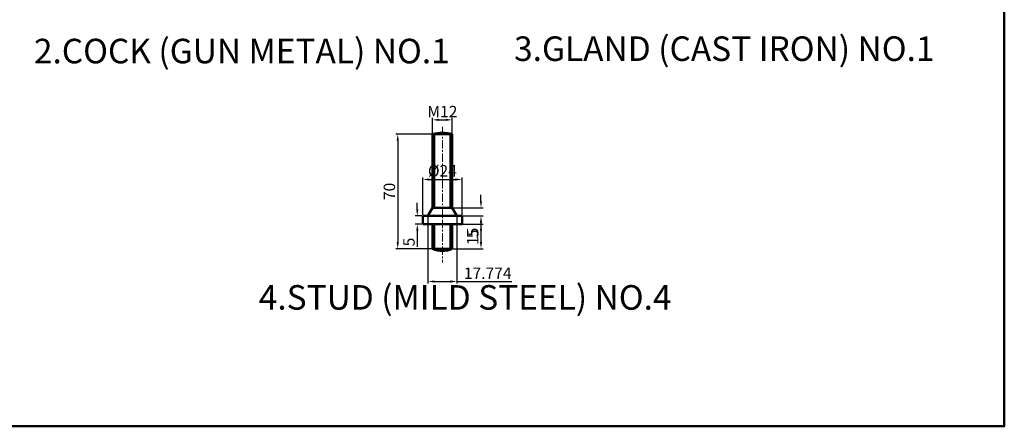
# Model space of a CAD drawing. Units: millimetres. Extents: x 49 to 1001, y -335 to 311.
# Tile 3 of 4: x 399 to 1001, y -335 to -87. Entities that reach past the tile are written whole.
import ezdxf

# ---------------------------------------------------------------- set-up
doc = ezdxf.new("R2010")
doc.units = ezdxf.units.MM
doc.header["$LTSCALE"] = 0.4
doc.linetypes.add('CENTER', pattern=[50.8, 31.75, -6.35, 6.35, -6.35])
for name, color, linetype, lineweight in [('M-CNTR', 1, 'CENTER', 18), ('M-DIMS', 2, 'Continuous', 25), ('M-OUTL', 7, 'Continuous', 50), ('M-TEXT', 3, 'Continuous', 25)]:
    doc.layers.add(name, color=color, linetype=linetype, lineweight=lineweight)
doc.styles.get("Standard").update_dxf_attribs({"font": 'arial.ttf'})
doc.dimstyles.new('ISO-25', dxfattribs={"dimtxt": 7, "dimasz": 4, "dimexe": 1.25, "dimexo": 0.625, "dimtad": 1, "dimtxsty": 'Standard', "dimcen": 2.5, "dimadec": 0, "dimazin": 0, "dimtfac": 1, "dimtofl": 0, "dimtmove": 0, "dimatfit": 3, "dimfxl": 1, "dimarcsym": 0})

# ---------------------------------------------------------------- blocks, each defined once
blk = doc.blocks.new('*D53')
at = {"layer": 'Defpoints', "color": 0, "ltscale": 0.4, "transparency": 16777216}
for p in [(657.67, -156.49), (630.35, -226.49), (657.67, -226.49)]:
    blk.add_point(p, dxfattribs=at)
at = {"layer": 'M-DIMS', "color": 0, "lineweight": -2, "ltscale": 0.4, "transparency": 16777216}
for p, q in [((657.05, -156.49), (629.1, -156.49)), ((630.35, -160.49), (630.35, -222.49)), ((657.05, -226.49), (629.1, -226.49))]:
    blk.add_line(p, q, dxfattribs=at)
at = {"layer": 'M-DIMS', "color": 0, "ltscale": 0.4, "transparency": 16777216}
for points in [[(629.68, -160.49), (631.02, -160.49), (630.35, -156.49)], [(629.68, -222.49), (631.02, -222.49), (630.35, -226.49)]]:
    blk.add_solid(points, dxfattribs=at)
at = {"layer": 'M-DIMS', "color": 0, "ltscale": 0.4, "transparency": 16777216, "insert": (626.15, -191.49), "char_height": 7, "attachment_point": 5, "rotation": 90}
blk.add_mtext('70', dxfattribs=at)
blk = doc.blocks.new('*D54')
at = {"layer": 'Defpoints', "color": 0, "ltscale": 0.4, "transparency": 16777216}
for p in [(645.67, -206.49), (642.31, -211.49), (645.67, -211.49)]:
    blk.add_point(p, dxfattribs=at)
at = {"layer": 'M-DIMS', "color": 0, "lineweight": -2, "ltscale": 0.4, "transparency": 16777216}
for p, q in [((642.31, -202.49), (642.31, -198.49)), ((645.05, -206.49), (641.06, -206.49)), ((645.05, -211.49), (641.06, -211.49)), ((642.31, -215.49), (642.31, -225.38))]:
    blk.add_line(p, q, dxfattribs=at)
at = {"layer": 'M-DIMS', "color": 0, "ltscale": 0.4, "transparency": 16777216}
for points in [[(641.64, -202.49), (642.97, -202.49), (642.31, -206.49)], [(641.64, -215.49), (642.97, -215.49), (642.31, -211.49)]]:
    blk.add_solid(points, dxfattribs=at)
at = {"layer": 'M-DIMS', "color": 0, "ltscale": 0.4, "transparency": 16777216, "insert": (638.12, -222.43), "char_height": 7, "attachment_point": 5, "rotation": 90}
blk.add_mtext('5', dxfattribs=at)
blk = doc.blocks.new('*D55')
at = {"layer": 'Defpoints', "color": 0, "ltscale": 0.4, "transparency": 16777216}
for p in [(669.67, -184.21), (645.67, -206.49), (669.67, -206.49)]:
    blk.add_point(p, dxfattribs=at)
at = {"layer": 'M-DIMS', "color": 0, "lineweight": -2, "ltscale": 0.4, "transparency": 16777216}
for p, q in [((645.67, -205.86), (645.67, -182.96)), ((649.67, -184.21), (665.67, -184.21)), ((669.67, -205.86), (669.67, -182.96))]:
    blk.add_line(p, q, dxfattribs=at)
at = {"layer": 'M-DIMS', "color": 0, "ltscale": 0.4, "transparency": 16777216}
for points in [[(649.67, -183.54), (649.67, -184.87), (645.67, -184.21)], [(665.67, -183.54), (665.67, -184.87), (669.67, -184.21)]]:
    blk.add_solid(points, dxfattribs=at)
at = {"layer": 'M-DIMS', "color": 0, "ltscale": 0.4, "transparency": 16777216, "insert": (657.67, -179.81), "char_height": 7, "attachment_point": 5}
blk.add_mtext('%%C24', dxfattribs=at)
blk = doc.blocks.new('*D56')
at = {"layer": 'Defpoints', "color": 0, "ltscale": 0.4, "transparency": 16777216}
for p in [(663.67, -147.74), (651.67, -164.1), (663.67, -164.1)]:
    blk.add_point(p, dxfattribs=at)
at = {"layer": 'M-DIMS', "color": 0, "lineweight": -2, "ltscale": 0.4, "transparency": 16777216}
for p, q in [((651.67, -163.48), (651.67, -146.49)), ((655.67, -147.74), (659.67, -147.74)), ((663.67, -163.48), (663.67, -146.49))]:
    blk.add_line(p, q, dxfattribs=at)
at = {"layer": 'M-DIMS', "color": 0, "ltscale": 0.4, "transparency": 16777216}
for points in [[(655.67, -147.08), (655.67, -148.41), (651.67, -147.74)], [(659.67, -147.08), (659.67, -148.41), (663.67, -147.74)]]:
    blk.add_solid(points, dxfattribs=at)
at = {"layer": 'M-DIMS', "color": 0, "ltscale": 0.4, "transparency": 16777216, "insert": (657.67, -143.6), "char_height": 7, "attachment_point": 5}
blk.add_mtext('M12', dxfattribs=at)
blk = doc.blocks.new('*D68')
at = {"layer": 'Defpoints', "color": 0, "ltscale": 0.4, "transparency": 16777216}
for p in [(663.67, -211.49), (663.67, -226.49), (681.27, -226.49)]:
    blk.add_point(p, dxfattribs=at)
at = {"layer": 'M-DIMS', "color": 0, "lineweight": -2, "ltscale": 0.4, "transparency": 16777216}
for p, q in [((664.3, -211.49), (682.52, -211.49)), ((681.27, -215.49), (681.27, -222.49)), ((664.3, -226.49), (682.52, -226.49))]:
    blk.add_line(p, q, dxfattribs=at)
at = {"layer": 'M-DIMS', "color": 0, "ltscale": 0.4, "transparency": 16777216}
for points in [[(680.61, -215.49), (681.94, -215.49), (681.27, -211.49)], [(680.61, -222.49), (681.94, -222.49), (681.27, -226.49)]]:
    blk.add_solid(points, dxfattribs=at)
at = {"layer": 'M-DIMS', "color": 0, "ltscale": 0.4, "transparency": 16777216, "insert": (677.08, -218.99), "char_height": 7, "attachment_point": 5, "rotation": 90}
blk.add_mtext('15', dxfattribs=at)
blk = doc.blocks.new('*D69')
at = {"layer": 'Defpoints', "color": 0, "ltscale": 0.4, "transparency": 16777216}
for p in [(663.67, -201.49), (666.56, -206.49), (681.27, -206.49)]:
    blk.add_point(p, dxfattribs=at)
at = {"layer": 'M-DIMS', "color": 0, "lineweight": -2, "ltscale": 0.4, "transparency": 16777216}
for p, q in [((681.27, -197.49), (681.27, -193.49)), ((664.3, -201.49), (682.52, -201.49)), ((667.19, -206.49), (682.52, -206.49)), ((681.27, -210.49), (681.27, -220.38))]:
    blk.add_line(p, q, dxfattribs=at)
at = {"layer": 'M-DIMS', "color": 0, "ltscale": 0.4, "transparency": 16777216}
for points in [[(680.61, -197.49), (681.94, -197.49), (681.27, -201.49)], [(680.61, -210.49), (681.94, -210.49), (681.27, -206.49)]]:
    blk.add_solid(points, dxfattribs=at)
at = {"layer": 'M-DIMS', "color": 0, "ltscale": 0.4, "transparency": 16777216, "insert": (677.09, -217.43), "char_height": 7, "attachment_point": 5, "rotation": 90}
blk.add_mtext('5', dxfattribs=at)
blk = doc.blocks.new('*D70')
at = {"layer": 'Defpoints', "color": 0, "ltscale": 0.4, "transparency": 16777216}
for p in [(648.79, -206.49), (666.56, -206.49), (666.56, -246.55)]:
    blk.add_point(p, dxfattribs=at)
at = {"layer": 'M-DIMS', "color": 0, "lineweight": -2, "ltscale": 0.4, "transparency": 16777216}
for p, q in [((648.79, -207.11), (648.79, -247.8)), ((666.56, -207.11), (666.56, -247.8)), ((652.79, -246.55), (662.56, -246.55)), ((666.56, -246.55), (700.18, -246.55))]:
    blk.add_line(p, q, dxfattribs=at)
at = {"layer": 'M-DIMS', "color": 0, "ltscale": 0.4, "transparency": 16777216}
for points in [[(652.79, -245.88), (652.79, -247.21), (648.79, -246.55)], [(662.56, -245.88), (662.56, -247.21), (666.56, -246.55)]]:
    blk.add_solid(points, dxfattribs=at)
at = {"layer": 'M-DIMS', "color": 0, "ltscale": 0.4, "transparency": 16777216, "insert": (685.37, -242.41), "char_height": 7, "attachment_point": 5}
blk.add_mtext('17.774', dxfattribs=at)

msp = doc.modelspace()

# ---------------------------------------------------------------- linework, layer by layer
at = {"layer": 'M-CNTR', "ltscale": 0.4}
msp.add_line((657.6741, -152.0482), (657.6741, -234.9461), dxfattribs=at)
at = {"layer": 'M-OUTL', "ltscale": 0.4}
for p, q in [((651.6741, -156.4864), (663.6741, -156.4864)), ((651.6741, -201.4864), (651.6741, -156.4864)), ((652.6741, -201.4864), (652.6741, -156.4864)), ((662.6741, -156.4864), (662.6741, -201.4864)), ((663.6741, -156.4864), (663.6741, -201.4864)), ((651.6741, -201.4864), (648.7873, -206.4864)), ((663.6741, -201.4864), (651.6741, -201.4864)), ((663.6741, -201.4864), (666.5608, -206.4864)), ((645.6741, -211.4864), (645.6741, -206.4864)), ((669.6741, -206.4864), (645.6741, -206.4864)), ((669.6741, -211.4864), (669.6741, -206.4864)), ((669.6741, -211.4864), (645.6741, -211.4864)), ((651.6741, -226.4864), (651.6741, -211.4864)), ((652.6741, -226.4864), (652.6741, -211.4864)), ((662.6741, -211.4864), (662.6741, -226.4864)), ((663.6741, -211.4864), (663.6741, -226.4864)), ((663.6741, -226.4864), (651.6741, -226.4864))]:
    msp.add_line(p, q, dxfattribs=at)
msp.add_lwpolyline([(48.6466, 311.3462), (1001.3348, 311.3462), (1001.3348, -335.0483), (48.6466, -335.0483)], close=True, dxfattribs=at)
for centre, radius, start, end in [((657.6741, -179.7138), 23.9898, 75.5162285, 104.4837715), ((657.6741, -214.2009), 13.6724, 243.9700246, 296.0299754)]:
    msp.add_arc(centre, radius, start, end, dxfattribs=at)

# ---------------------------------------------------------------- texts
at = {"layer": 'M-TEXT', "ltscale": 0.4, "char_height": 15, "attachment_point": 1}
for s, insert in [('3.GLAND (CAST IRON) NO.1', (701.5145, -96.7373)), ('2.COCK (GUN METAL) NO.1', (407.8459, -98.1839)), ('4.STUD (MILD STEEL) NO.4', (545.3697, -248.7571))]:
    msp.add_mtext_dynamic_manual_height_columns(s, width=273.753282, gutter_width=12.5, heights=[0], dxfattribs=dict(at, insert=insert))

# ---------------------------------------------------------------- dimensions: what is measured, and where the dimension line sits
at = {"layer": 'M-DIMS', "ltscale": 0.4}
dim = msp.add_linear_dim(base=(663.6741, -147.7435), p1=(651.6741, -164.1042), p2=(663.6741, -164.1042), text='M<>', dimstyle='ISO-25', override={"dimclrd": 0, "dimclre": 0, "dimclrt": 0}, dxfattribs=at)
dim.commit()
dim.dimension.update_dxf_attribs({"geometry": '*D56', "text_midpoint": (657.6741, -147.7435), "dimtype": 160})
for base, p1, p2, override, picture, middle in [((630.3509, -226.4864), (657.6741, -156.4864), (657.6741, -226.4864), {"dimclrd": 0, "dimclre": 0, "dimclrt": 0}, '*D53', (626.1519, -191.4864)), ((642.3061, -211.4864), (645.6741, -206.4864), (645.6741, -211.4864), {"dimclrd": 0, "dimclre": 0, "dimclrt": 0}, '*D54', (638.1214, -222.432)), ((681.2741, -206.4864), (663.6741, -201.4864), (666.5608, -206.4864), {"dimdec": 0, "dimlfac": 1, "dimrnd": 0, "dimzin": 0, "dimdsep": 46, "dimlunit": 2}, '*D69', (677.0894, -217.432)), ((681.2741, -226.4864), (663.6741, -211.4864), (663.6741, -226.4864), {"dimdec": 0, "dimlfac": 1, "dimrnd": 0, "dimzin": 0, "dimdsep": 46, "dimlunit": 2}, '*D68', (677.0751, -218.9864))]:
    dim = msp.add_linear_dim(base=base, p1=p1, p2=p2, angle=90, dimstyle='ISO-25', override=override, dxfattribs=at)
    dim.commit()
    dim.dimension.update_dxf_attribs({"geometry": picture, "text_midpoint": middle})
dim = msp.add_linear_dim(base=(669.6741, -184.2073), p1=(645.6741, -206.4864), p2=(669.6741, -206.4864), text='%%C<>', dimstyle='ISO-25', override={"dimclrd": 0, "dimclre": 0, "dimclrt": 0}, dxfattribs=at)
dim.commit()
dim.dimension.update_dxf_attribs({"geometry": '*D55', "text_midpoint": (657.6741, -179.8125)})
dim = msp.add_linear_dim(base=(666.560818, -246.546149), p1=(648.787315, -206.486382), p2=(666.560818, -206.486382), dimstyle='ISO-25', override={"dimdec": 3, "dimlfac": 1, "dimrnd": 0, "dimzin": 0, "dimdsep": 46, "dimlunit": 2}, dxfattribs=at)
dim.commit()
dim.dimension.update_dxf_attribs({"geometry": '*D70', "text_midpoint": (685.372039, -242.406824)})

doc.saveas('drawing.dxf')
